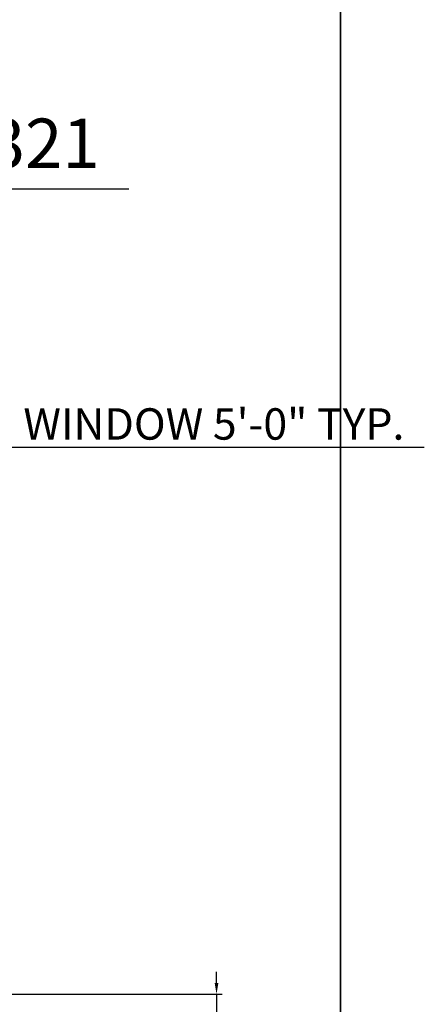
# Model space of a CAD drawing. Units: inches. Extents: x 1484 to 2008, y 1843 to 2590.
# Tile 20 of 21: x 1918 to 2008, y 2075 to 2295. Entities that reach past the tile are written whole.
import ezdxf

# ---------------------------------------------------------------- set-up
doc = ezdxf.new("R2010")
doc.units = ezdxf.units.IN
for name, color, linetype, lineweight in [('A-ANNO-DIMS', 2, 'Continuous', 18), ('A-ANNO-TEXT', 7, 'Continuous', 25), ('A-ANNO-TTLB', 7, 'Continuous', 35)]:
    doc.layers.add(name, color=color, linetype=linetype, lineweight=lineweight)
doc.styles.get("Standard").update_dxf_attribs({"font": 'arial.ttf'})
doc.dimstyles.new('ISO-25', dxfattribs={"dimtxt": 7, "dimasz": 2.5, "dimexe": 1.25, "dimexo": 0.625, "dimtad": 1, "dimdec": 0, "dimlunit": 3, "dimtxsty": 'Standard', "dimcen": 2.5, "dimadec": 0, "dimazin": 0, "dimtfac": 1, "dimtdec": 0, "dimtmove": 0, "dimatfit": 3, "dimfxl": 1, "dimarcsym": 0})

# ---------------------------------------------------------------- blocks, each defined once
blk = doc.blocks.new('*D13')
at = {"layer": 'A-ANNO-DIMS', "color": 0, "lineweight": -2, "transparency": 16777216}
for p, q in [((1803.22, 2207.68), (1803.22, 2198.05)), ((1863.22, 2207.68), (1863.22, 2198.05)), ((1805.72, 2199.3), (1860.72, 2199.3)), ((1863.22, 2199.3), (2008.2, 2199.3))]:
    blk.add_line(p, q, dxfattribs=at)
at = {"layer": 'A-ANNO-DIMS', "color": 0, "transparency": 16777216}
for points in [[(1805.72, 2199.72), (1805.72, 2198.89), (1803.22, 2199.3)], [(1860.72, 2199.72), (1860.72, 2198.89), (1863.22, 2199.3)]]:
    blk.add_solid(points, dxfattribs=at)
at = {"layer": 'Defpoints', "color": 0, "transparency": 16777216}
for p in [(1803.22, 2208.3), (1863.22, 2208.3), (1863.22, 2199.3)]:
    blk.add_point(p, dxfattribs=at)
at = {"layer": 'A-ANNO-DIMS', "color": 0, "transparency": 16777216, "insert": (1936.96, 2203.55), "char_height": 7, "attachment_point": 5}
blk.add_mtext('BEDROOM WINDOW 5\'-0" TYP.', dxfattribs=at)
blk = doc.blocks.new('*D41')
at = {"layer": 'A-ANNO-DIMS', "color": 0, "lineweight": -2, "transparency": 16777216}
for p, q in [((1961.85, 2079.8), (1961.85, 2082.3)), ((1891.54, 2077.3), (1963.1, 2077.3)), ((1961.85, 2077.3), (1961.85, 2072.8)), ((1891.54, 2072.8), (1963.1, 2072.8)), ((1961.85, 2070.3), (1961.85, 2031.63))]:
    blk.add_line(p, q, dxfattribs=at)
at = {"layer": 'A-ANNO-DIMS', "color": 0, "transparency": 16777216}
for points in [[(1961.44, 2079.8), (1962.27, 2079.8), (1961.85, 2077.3)], [(1961.44, 2070.3), (1962.27, 2070.3), (1961.85, 2072.8)]]:
    blk.add_solid(points, dxfattribs=at)
at = {"layer": 'Defpoints', "color": 0, "transparency": 16777216}
for p in [(1890.92, 2077.3), (1890.92, 2072.8), (1961.85, 2072.8)]:
    blk.add_point(p, dxfattribs=at)
at = {"layer": 'A-ANNO-DIMS', "color": 0, "transparency": 16777216, "insert": (1957.61, 2049.72), "char_height": 7, "attachment_point": 5, "rotation": 90}
blk.add_mtext('0\'-4 1/2"', dxfattribs=at)

msp = doc.modelspace()

# ---------------------------------------------------------------- linework, layer by layer
at = {"layer": 'A-ANNO-TEXT'}
msp.add_line((1588.86, 2256.92), (1942.3, 2256.92), dxfattribs=at)
at = {"layer": 'A-ANNO-TTLB'}
msp.add_lwpolyline([(1484.04, 2590.09), (1989.53, 2590.09), (1989.53, 1843.34), (1484.04, 1843.34)], close=True, dxfattribs=at)

# ---------------------------------------------------------------- texts
at = {"layer": 'A-ANNO-TEXT', "insert": (1591.11, 2272.55), "char_height": 11, "attachment_point": 1}
msp.add_mtext_dynamic_manual_height_columns('25X25 [625 sq ft ] House Plan -North face - FP1321', width=378.3718, gutter_width=12.5, heights=[0], dxfattribs=at)

# ---------------------------------------------------------------- dimensions: what is measured, and where the dimension line sits
at = {"layer": 'A-ANNO-DIMS'}
dim = msp.add_linear_dim(base=(1863.22, 2199.3), p1=(1803.22, 2208.3), p2=(1863.22, 2208.3), text='BEDROOM WINDOW <> TYP.', dimstyle='ISO-25', override={"dimdec": 1, "dimlfac": 1, "dimrnd": 0, "dimzin": 1, "dimdsep": 46, "dimlunit": 4, "dimfrac": 2}, dxfattribs=at)
dim.commit()
dim.dimension.update_dxf_attribs({"geometry": '*D13', "text_midpoint": (1936.96, 2203.55)})
dim = msp.add_linear_dim(base=(1961.85, 2072.8), p1=(1890.92, 2077.3), p2=(1890.92, 2072.8), angle=90, dimstyle='ISO-25', override={"dimdec": 1, "dimlfac": 1, "dimrnd": 0, "dimzin": 1, "dimdsep": 46, "dimlunit": 4, "dimfrac": 2}, dxfattribs=at)
dim.commit()
dim.dimension.update_dxf_attribs({"geometry": '*D41', "text_midpoint": (1957.61, 2049.72)})

doc.saveas('drawing.dxf')
